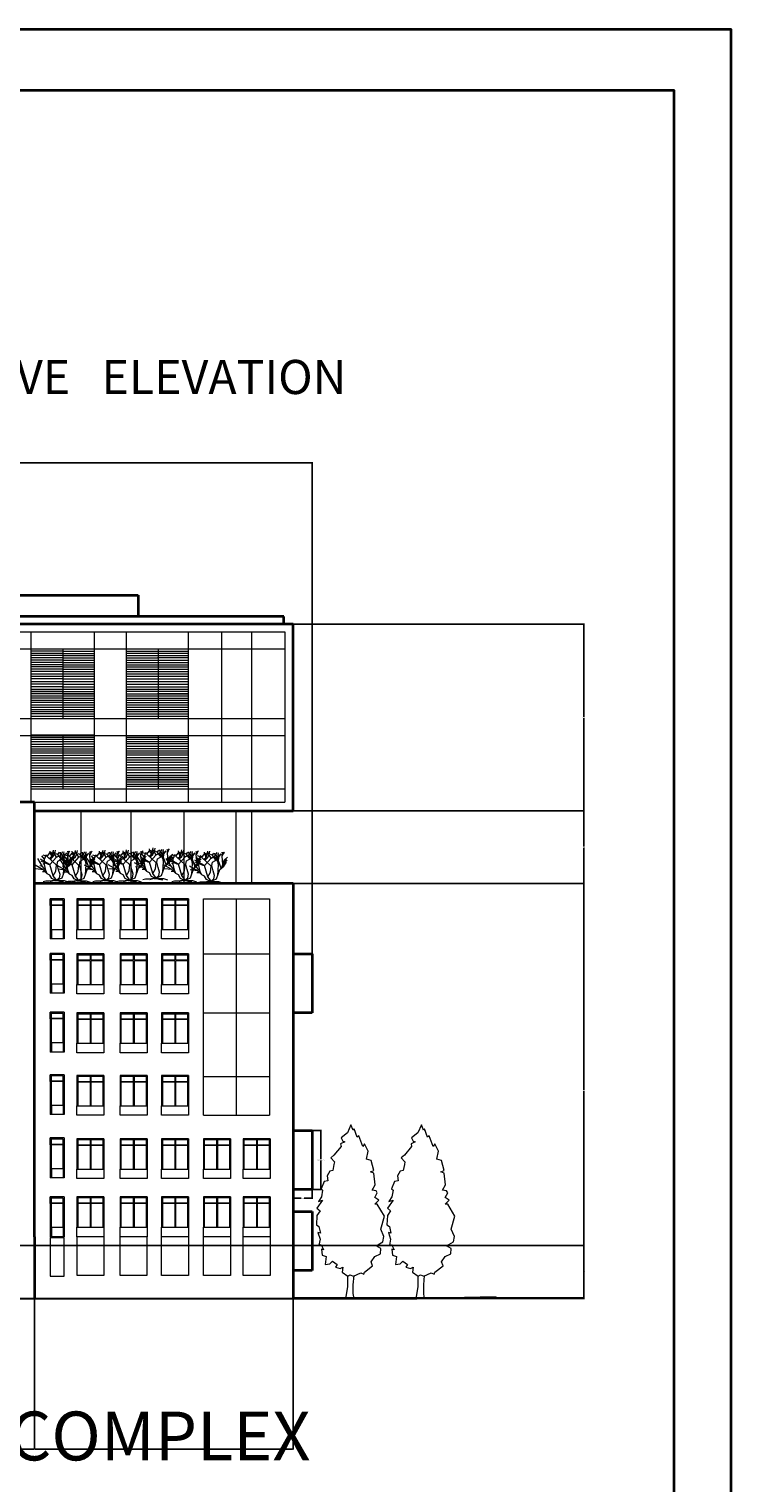
# Model space of a CAD drawing. Units: inches. Extents: x -279 to 364, y -385 to 335.
# Tile 9 of 9: x 168 to 364, y -72 to 335. Entities that reach past the tile are written whole.
import ezdxf

# ---------------------------------------------------------------- set-up
doc = ezdxf.new("R2010")
doc.units = ezdxf.units.IN
doc.header["$MEASUREMENT"] = 0
for name, color, linetype, lineweight in [('A-ANNO-DIMS', 2, 'Continuous', 18), ('A-ANNO-TEXT', 7, 'Continuous', 25), ('A-ANNO-TTLB', 7, 'Continuous', 35), ('A-GLAZ', 4, 'Continuous', 18), ('A-GLAZ-CURT', 4, 'Continuous', 18), ('A-ROOF', 7, 'Continuous', 35), ('A-WALL', 7, 'Continuous', 35), ('A-WALL-LOUV', 8, 'Continuous', 13), ('C-TOPO', 32, 'Continuous', 30), ('L-PLNT', 94, 'Continuous', 13)]:
    doc.layers.add(name, color=color, linetype=linetype, lineweight=lineweight)
doc.styles.get("Standard").update_dxf_attribs({"font": 'arial.ttf'})
doc.dimstyles.get("Standard").update_dxf_attribs({"dimtxt": 0.18, "dimasz": 0.18, "dimexe": 0.18, "dimexo": 0.0625, "dimgap": 0.09, "dimtad": 0, "dimtih": 1, "dimtoh": 1, "dimdec": 4, "dimzin": 0, "dimdsep": 46, "dimtxsty": 'Standard', "dimcen": 0.09, "dimadec": 0, "dimazin": 0, "dimtfac": 1, "dimtdec": 4, "dimtofl": 0, "dimtmove": 0, "dimatfit": 3, "dimfxl": 1, "dimtolj": 1, "dimtzin": 0, "dimarcsym": 0})

# ---------------------------------------------------------------- blocks, each defined once
blk = doc.blocks.new('*U2')
for p, q in [((-12.471, 19.775), (-12.898, 22.044)), ((-11.28, 19.619), (-12.104, 21.184)), ((-11.433, 18.289), (-10.457, 22.749)), ((-8.16, 17.76), (-10.56, 21.6)), ((-9.48, 19.775), (-8.992, 22.592)), ((-7.2, 19.68), (-6.24, 21.12)), ((-5.086, 17.741), (-5.513, 21.34)), ((-5.28, 19.2), (-3.84, 21.6)), ((-3.377, 18.602), (-2.888, 21.575)), ((-0.508, 21.888), (-0.081, 20.558)), ((-0.203, 19.149), (0.102, 21.34)), ((-0.02, 20.01), (0.896, 21.105)), ((0.041, 20.714), (1.384, 22.044)), ((0.102, 21.34), (0.835, 21.888)), ((-17.76, 8.64), (-23.663, 11.961)), ((-18.24, 11.04), (-21.755, 16.655)), ((-18.24, 11.04), (-20.16, 11.52)), ((-12.96, 12.48), (-19.68, 16.32)), ((-13.92, 12.48), (-19.2, 14.88)), ((-16.8, 16.32), (-18.72, 18.72)), ((-15.84, 8.16), (-18.24, 11.04)), ((-14.88, 18.24), (-17.76, 19.2)), ((-16.8, 12.48), (-17.76, 12.96)), ((-16.8, 16.32), (-15.36, 19.68)), ((-16.8, 12.48), (-16.8, 16.32)), ((-15.84, 8.16), (-16.8, 12.48)), ((-14.88, 18.24), (-12.96, 20.64)), ((-8.16, 12), (-14.88, 18.24)), ((-12.96, 12.48), (-13.92, 12.48)), ((-13.325, 16.724), (-11.433, 18.289)), ((-12.96, 12.48), (-8.16, 17.76)), ((-10.56, 4.32), (-12.96, 12.48)), ((-11.677, 19.071), (-12.471, 19.775)), ((-12.043, 15.628), (-11.921, 18.836)), ((-11.982, 16.802), (-10.579, 18.054)), ((-11.921, 18.836), (-10.64, 20.401)), ((-10.579, 18.054), (-9.846, 19.697)), ((-7.2, 19.68), (-8.64, 20.16)), ((-8.64, 7.68), (-8.16, 12)), ((-8.16, 17.76), (-5.28, 19.2)), ((-7.68, 12.48), (-7.2, 14.88)), ((-6.72, 8.64), (-7.68, 12.48)), ((-4.8, 16.32), (-7.2, 19.68)), ((-7.2, 14.88), (-3.84, 16.8)), ((-3.377, 15.315), (-5.086, 17.819)), ((-2.88, 12.96), (-4.32, 19.68)), ((-3.84, 16.8), (-0.96, 20.64)), ((-2.766, 16.802), (-3.377, 18.602)), ((-3.36, 5.28), (-2.88, 12.96)), ((-2.88, 15.84), (-2.4, 20.16)), ((-0.96, 10.56), (-2.88, 15.84)), ((-1.92, 9.6), (0.96, 12)), ((-0.48, 10.8), (0.346, 13.203)), ((0.346, 13.203), (-0.203, 19.149)), ((-0.142, 19.384), (0.59, 20.401)), ((0.346, 13.203), (1.323, 16.254)), ((0.96, 12), (1.44, 15.36)), ((0.96, 12), (2.88, 14.88)), ((1.323, 16.254), (3.642, 18.289)), ((1.44, 15.36), (2.88, 17.28)), ((1.92, 13.44), (2.4, 15.36)), ((2.4, 15.36), (3.36, 16.32)), ((-17.76, 8.64), (-23.128, 9.222)), ((-16.32, 7.2), (-18.24, 7.2)), ((-14.88, 5.76), (-17.76, 8.64)), ((-15.84, 0.48), (-17.76, 0)), ((-14.88, 5.76), (-15.84, 8.16)), ((-13.44, 0.48), (-15.84, 0.48)), ((-12.96, 4.8), (-14.88, 5.76)), ((-9.6, 0.96), (-13.44, 0.48)), ((-11.52, 2.4), (-12.96, 4.8)), ((-9.6, 0.96), (-12.96, 0)), ((-8.64, 0.96), (-11.52, 2.4)), ((-10.56, 4.32), (-8.64, 7.68)), ((-8.64, 1.92), (-10.56, 4.32)), ((-9.6, 0.96), (-7.68, 0.96)), ((-8.64, 0.96), (-4.32, 2.88)), ((-8.64, 0.96), (-6.24, 2.88)), ((-8.64, 0.96), (-8.64, 1.92)), ((-8.64, 0.96), (-2.88, 0.96)), ((-7.68, 0.96), (-6.24, 0.48)), ((-5.76, 5.28), (-6.72, 8.64)), ((-6.24, 2.88), (-5.76, 5.28)), ((-6.24, 0.48), (-3.36, 0)), ((-4.32, 2.88), (-1.92, 9.6)), ((-2.88, 0.96), (0, 0))]:
    blk.add_line(p, q)
blk = doc.blocks.new('*U3')
blk.add_lwpolyline([(-2.754, 191.699), (-6.78, 182.851), (-13.682, 176.953), (-11.956, 173.266), (-9.656, 172.529), (-14.257, 170.317), (-13.682, 167.368), (-21.733, 157.783), (-25.184, 154.834), (-21.158, 150.41), (-21.733, 147.461), (-22.884, 140.825), (-26.334, 140.087), (-29.21, 134.926), (-28.635, 129.028), (-32.661, 128.291), (-36.111, 120.18), (-34.386, 118.706), (-35.536, 111.333), (-38.987, 106.171), (-34.386, 107.646), (-40.712, 98.798), (-37.261, 95.849), (-40.712, 90.688), (-41.287, 80.366), (-38.412, 78.154), (-36.686, 70.781), (-39.562, 71.518), (-37.261, 64.145), (-38.412, 57.509), (-36.111, 58.247), (-33.236, 52.348), (-35.536, 53.086), (-34.961, 46.45), (-30.36, 44.975), (-31.51, 36.128), (-26.334, 36.865), (-23.459, 39.814), (-18.283, 36.128), (-20.008, 33.178), (-14.832, 31.704), (-11.956, 33.178), (-12.531, 27.28), (-6.205, 22.856), (-3.905, 24.331), (0.121, 22.856), (8.173, 26.543), (11.624, 25.068), (12.199, 27.28), (21.4, 34.653), (19.675, 39.077), (23.701, 44.975), (30.027, 47.924), (30.602, 53.823), (25.426, 56.772), (32.903, 61.196), (34.053, 67.094), (30.602, 75.205), (34.628, 89.951), (26.576, 103.222), (23.701, 103.222), (28.302, 107.646), (23.701, 110.595), (26.576, 115.756), (25.426, 117.968), (20.825, 118.706), (24.276, 124.604), (22.551, 137.876), (19.1, 139.35), (22.551, 140.825), (19.675, 151.884), (14.499, 153.359), (16.224, 162.207), (12.199, 170.317), (10.473, 167.368), (5.872, 179.165), (4.147, 177.69), (0.696, 187.275), (-0.454, 185.8)], close=True)
for points in [[(-6.813, 23.669), (-6.813, 11.669), (-8.627, 0)], [(0.387, 23.669), (-0.576, 13.271), (-0.576, 3.686), (0, 0)]]:
    blk.add_lwpolyline(points)
blk = doc.blocks.new('WIN-WING-NARROW')
for p, q in [((0, 11.12), (0, 0)), ((0, 11.12), (3.85, 11.12)), ((0.2, 2.62), (0.2, 10.81)), ((0.2, 10.81), (3.85, 10.81)), ((0.2, 9.34), (3.52, 9.34)), ((0.2, 9.24), (3.52, 9.24)), ((3.52, 9.34), (3.52, 10.81)), ((3.52, 2.62), (3.52, 9.24)), ((3.85, 9.24), (3.85, 11.12)), ((3.85, 10.81), (3.85, 9.34)), ((3.85, 9.24), (3.85, 2.62)), ((3.85, 2.62), (0, 2.62)), ((0, 0), (3.85, 0)), ((0.2, 2.62), (0.2, 0)), ((3.52, 2.62), (3.52, 0)), ((3.85, 2.62), (3.85, 0))]:
    blk.add_line(p, q)
blk = doc.blocks.new('WING-RETURN-LONG')
for p, q in [((0, 16.47), (5.32, 16.47)), ((5.32, 16.47), (5.32, 0)), ((5.32, 0), (0, 0))]:
    blk.add_line(p, q)
blk = doc.blocks.new('WIN-WING-TWIN')
for p, q in [((0, 11.12), (0, 0)), ((0, 11.12), (7.53, 11.12)), ((0.2, 2.62), (0.2, 10.81)), ((0.2, 10.81), (7.32, 10.81)), ((0.2, 9.34), (3.52, 9.34)), ((0.2, 9.24), (3.52, 9.24)), ((3.52, 9.34), (3.52, 10.81)), ((3.52, 2.62), (3.52, 9.24)), ((3.85, 10.81), (3.85, 9.34)), ((3.85, 9.34), (7.32, 9.34)), ((3.85, 9.24), (7.32, 9.24)), ((3.85, 9.24), (3.85, 2.62)), ((7.32, 10.81), (7.32, 2.62)), ((7.53, 11.12), (7.53, 2.62)), ((7.53, 2.62), (0, 2.62)), ((0, 0), (7.53, 0)), ((7.53, 0), (7.53, 2.62))]:
    blk.add_line(p, q)
blk = doc.blocks.new('*D66')
at = {"layer": 'A-ANNO-DIMS', "color": 0, "lineweight": -2, "transparency": 16777216}
for p, q in [((246.99, 26.91), (249.58, 26.91)), ((249.4, 26.73), (249.4, 18.86)), ((249.4, 10.62), (249.4, 18.49)), ((246.99, 10.44), (249.58, 10.44))]:
    blk.add_line(p, q, dxfattribs=at)
at = {"layer": 'A-ANNO-DIMS', "color": 0, "transparency": 16777216}
for points in [[(249.37, 26.73), (249.43, 26.73), (249.4, 26.91)], [(249.37, 10.62), (249.43, 10.62), (249.4, 10.44)]]:
    blk.add_solid(points, dxfattribs=at)
at = {"layer": 'Defpoints', "color": 0, "transparency": 16777216}
for p in [(246.93, 26.91), (249.4, 26.91), (246.93, 10.44)]:
    blk.add_point(p, dxfattribs=at)
at = {"layer": 'A-ANNO-DIMS', "color": 0, "transparency": 16777216, "insert": (249.4, 18.67), "char_height": 0.18, "attachment_point": 5}
blk.add_mtext('\\A1;RETURN 16 TYP.', dxfattribs=at)
blk = doc.blocks.new('*D67')
at = {"layer": 'A-ANNO-DIMS', "color": 0, "lineweight": -2, "transparency": 16777216}
for p, q in [((241.6, 10.38), (241.6, 7.79)), ((246.93, 10.38), (246.93, 7.79)), ((241.78, 7.97), (243.81, 7.97)), ((246.75, 7.97), (244.72, 7.97))]:
    blk.add_line(p, q, dxfattribs=at)
at = {"layer": 'A-ANNO-DIMS', "color": 0, "transparency": 16777216}
for points in [[(241.78, 8), (241.78, 7.94), (241.6, 7.97)], [(246.75, 8), (246.75, 7.94), (246.93, 7.97)]]:
    blk.add_solid(points, dxfattribs=at)
at = {"layer": 'Defpoints', "color": 0, "transparency": 16777216}
for p in [(241.6, 10.44), (246.93, 10.44), (246.93, 7.97)]:
    blk.add_point(p, dxfattribs=at)
at = {"layer": 'A-ANNO-DIMS', "color": 0, "transparency": 16777216, "insert": (244.26, 7.97), "char_height": 0.18, "attachment_point": 5}
blk.add_mtext('\\A1;5 TYP.', dxfattribs=at)
blk = doc.blocks.new('*D74')
at = {"layer": 'A-ANNO-DIMS', "color": 0, "lineweight": -2, "transparency": 16777216}
for p, q in [((-137.56, 76.08), (-137.56, 213.67)), ((-137.38, 213.49), (54.29, 213.49)), ((246.75, 213.49), (55.08, 213.49)), ((246.93, 76.27), (246.93, 213.67))]:
    blk.add_line(p, q, dxfattribs=at)
at = {"layer": 'A-ANNO-DIMS', "color": 0, "transparency": 16777216}
for points in [[(-137.38, 213.52), (-137.38, 213.46), (-137.56, 213.49)], [(246.75, 213.52), (246.75, 213.46), (246.93, 213.49)]]:
    blk.add_solid(points, dxfattribs=at)
at = {"layer": 'Defpoints', "color": 0, "transparency": 16777216}
for p in [(246.93, 213.49), (-137.56, 76.01), (246.93, 76.21)]:
    blk.add_point(p, dxfattribs=at)
at = {"layer": 'A-ANNO-DIMS', "color": 0, "transparency": 16777216, "insert": (54.68, 213.49), "char_height": 0.18, "attachment_point": 5}
blk.add_mtext('\\A1;384.5', dxfattribs=at)
blk = doc.blocks.new('*D80')
at = {"layer": 'A-ANNO-DIMS', "color": 0, "lineweight": -2, "transparency": 16777216}
for p, q in [((94.22, -19.95), (94.22, -62.3)), ((169.29, -19.95), (169.29, -62.3)), ((94.4, -62.12), (131.36, -62.12)), ((169.11, -62.12), (132.15, -62.12))]:
    blk.add_line(p, q, dxfattribs=at)
at = {"layer": 'A-ANNO-DIMS', "color": 0, "transparency": 16777216}
for points in [[(94.4, -62.09), (94.4, -62.15), (94.22, -62.12)], [(169.11, -62.09), (169.11, -62.15), (169.29, -62.12)]]:
    blk.add_solid(points, dxfattribs=at)
at = {"layer": 'Defpoints', "color": 0, "transparency": 16777216}
for p in [(94.22, -19.89), (169.29, -19.89), (169.29, -62.12)]:
    blk.add_point(p, dxfattribs=at)
at = {"layer": 'A-ANNO-DIMS', "color": 0, "transparency": 16777216, "insert": (131.76, -62.12), "char_height": 0.18, "attachment_point": 5}
blk.add_mtext('\\A1;75.07', dxfattribs=at)
blk = doc.blocks.new('*D81')
at = {"layer": 'A-ANNO-DIMS', "color": 0, "lineweight": -2, "transparency": 16777216}
for p, q in [((169.29, -19.95), (169.29, -62.3)), ((241.6, -19.95), (241.6, -62.3)), ((169.47, -62.12), (205.07, -62.12)), ((241.42, -62.12), (205.82, -62.12))]:
    blk.add_line(p, q, dxfattribs=at)
at = {"layer": 'A-ANNO-DIMS', "color": 0, "transparency": 16777216}
for points in [[(169.47, -62.09), (169.47, -62.15), (169.29, -62.12)], [(241.42, -62.09), (241.42, -62.15), (241.6, -62.12)]]:
    blk.add_solid(points, dxfattribs=at)
at = {"layer": 'Defpoints', "color": 0, "transparency": 16777216}
for p in [(169.29, -19.89), (241.6, -19.89), (241.6, -62.12)]:
    blk.add_point(p, dxfattribs=at)
at = {"layer": 'A-ANNO-DIMS', "color": 0, "transparency": 16777216, "insert": (205.45, -62.12), "char_height": 0.18, "attachment_point": 5}
blk.add_mtext('\\A1;72.31', dxfattribs=at)
blk = doc.blocks.new('*D82')
at = {"layer": 'A-ANNO-DIMS', "color": 0, "lineweight": -2, "transparency": 16777216}
for p, q in [((241.67, 95.9), (323.06, 95.9)), ((322.88, 95.72), (322.88, 38.19)), ((322.88, -19.71), (322.88, 37.83)), ((241.67, -19.89), (323.06, -19.89))]:
    blk.add_line(p, q, dxfattribs=at)
at = {"layer": 'A-ANNO-DIMS', "color": 0, "transparency": 16777216}
for points in [[(322.85, 95.72), (322.91, 95.72), (322.88, 95.9)], [(322.85, -19.71), (322.91, -19.71), (322.88, -19.89)]]:
    blk.add_solid(points, dxfattribs=at)
at = {"layer": 'Defpoints', "color": 0, "transparency": 16777216}
for p in [(241.6, 95.9), (322.88, 95.9), (241.6, -19.89)]:
    blk.add_point(p, dxfattribs=at)
at = {"layer": 'A-ANNO-DIMS', "color": 0, "transparency": 16777216, "insert": (322.88, 38.01), "char_height": 0.18, "attachment_point": 5}
blk.add_mtext('\\A1;115.8', dxfattribs=at)
blk = doc.blocks.new('*D83')
at = {"layer": 'A-ANNO-DIMS', "color": 0, "lineweight": -2, "transparency": 16777216}
for p, q in [((241.67, 116.19), (323.06, 116.19)), ((322.88, 116.01), (322.88, 106.23)), ((322.88, 96.08), (322.88, 105.86)), ((241.67, 95.9), (323.06, 95.9))]:
    blk.add_line(p, q, dxfattribs=at)
at = {"layer": 'A-ANNO-DIMS', "color": 0, "transparency": 16777216}
for points in [[(322.85, 116.01), (322.91, 116.01), (322.88, 116.19)], [(322.85, 96.08), (322.91, 96.08), (322.88, 95.9)]]:
    blk.add_solid(points, dxfattribs=at)
at = {"layer": 'Defpoints', "color": 0, "transparency": 16777216}
for p in [(241.6, 116.19), (322.88, 116.19), (241.6, 95.9)]:
    blk.add_point(p, dxfattribs=at)
at = {"layer": 'A-ANNO-DIMS', "color": 0, "transparency": 16777216, "insert": (322.88, 106.05), "char_height": 0.18, "attachment_point": 5}
blk.add_mtext('\\A1;20.283', dxfattribs=at)
blk = doc.blocks.new('*D84')
at = {"layer": 'A-ANNO-DIMS', "color": 0, "lineweight": -2, "transparency": 16777216}
for p, q in [((241.67, 168.38), (323.06, 168.38)), ((322.88, 168.2), (322.88, 142.47)), ((322.88, 116.37), (322.88, 142.1)), ((241.67, 116.19), (323.06, 116.19))]:
    blk.add_line(p, q, dxfattribs=at)
at = {"layer": 'A-ANNO-DIMS', "color": 0, "transparency": 16777216}
for points in [[(322.85, 168.2), (322.91, 168.2), (322.88, 168.38)], [(322.85, 116.37), (322.91, 116.37), (322.88, 116.19)]]:
    blk.add_solid(points, dxfattribs=at)
at = {"layer": 'Defpoints', "color": 0, "transparency": 16777216}
for p in [(241.6, 168.38), (322.88, 168.38), (241.6, 116.19)]:
    blk.add_point(p, dxfattribs=at)
at = {"layer": 'A-ANNO-DIMS', "color": 0, "transparency": 16777216, "insert": (322.88, 142.28), "char_height": 0.18, "attachment_point": 5}
blk.add_mtext('\\A1;52.19', dxfattribs=at)
blk = doc.blocks.new('*D96')
at = {"layer": 'A-ANNO-DIMS', "color": 0, "lineweight": -2, "transparency": 16777216}
for p, q in [((76.18, -5.23), (323.06, -5.23)), ((322.88, -5.41), (322.88, -12.47)), ((322.88, -19.9), (322.88, -12.84)), ((75.75, -20.08), (323.06, -20.08))]:
    blk.add_line(p, q, dxfattribs=at)
at = {"layer": 'A-ANNO-DIMS', "color": 0, "transparency": 16777216}
for points in [[(322.85, -5.41), (322.91, -5.41), (322.88, -5.23)], [(322.85, -19.9), (322.91, -19.9), (322.88, -20.08)]]:
    blk.add_solid(points, dxfattribs=at)
at = {"layer": 'Defpoints', "color": 0, "transparency": 16777216}
for p in [(76.12, -5.23), (322.88, -5.23), (75.69, -20.08)]:
    blk.add_point(p, dxfattribs=at)
at = {"layer": 'A-ANNO-DIMS', "color": 0, "transparency": 16777216, "insert": (322.88, -12.66), "char_height": 0.18, "attachment_point": 5}
blk.add_mtext('\\A1;14.854', dxfattribs=at)

msp = doc.modelspace()

# ---------------------------------------------------------------- linework, layer by layer
at = {"layer": 'A-ANNO-TTLB'}
for points in [[(-279.2289, 334.6468), (364.0508, 334.6468), (364.0508, -385.2219), (-279.2289, -385.2219)], [(-267.2403, 317.5778), (348.1051, 317.5778), (348.1051, -370.8321), (-267.2403, -370.8321)]]:
    msp.add_lwpolyline(points, close=True, dxfattribs=at)
at = {"layer": 'A-GLAZ'}
for p, q in [((212.1476, 41.9776), (212.3516, 41.9776)), ((173.6886, -2.9883), (177.5344, -2.9883)), ((173.6886, -2.9883), (173.6886, -13.8647)), ((177.5344, -13.8647), (177.5344, -2.9883)), ((181.173, -13.6713), (181.173, -2.7885)), ((188.7012, -2.7885), (188.7012, -13.6713)), ((193.1921, -13.6713), (193.1921, -2.7885)), ((200.7203, -2.7885), (200.7203, -13.6713)), ((204.8183, -13.6713), (204.8183, -2.7885)), ((212.3465, -2.7885), (212.3465, -13.6713)), ((216.5376, -13.6713), (216.5376, -2.7885)), ((224.0658, -2.7885), (224.0658, -13.6713)), ((227.6488, -13.6713), (227.6488, -2.7885)), ((235.177, -2.7885), (235.177, -13.6713)), ((173.6886, -13.8647), (177.5344, -13.8647)), ((177.5344, -13.8647), (177.5344, -13.8647)), ((188.7012, -13.6713), (181.173, -13.6713)), ((200.7203, -13.6713), (193.1921, -13.6713)), ((212.3465, -13.6713), (204.8183, -13.6713)), ((224.0658, -13.6713), (216.5376, -13.6713)), ((235.177, -13.6713), (227.6488, -13.6713))]:
    msp.add_line(p, q, dxfattribs=at)
at = {"layer": 'A-GLAZ-CURT'}
for p, q in [((131.2105, 166.2338), (239.2791, 166.2338)), ((168.2851, 166.2338), (168.2851, 118.6379)), ((185.9755, 166.2338), (185.9755, 118.6379)), ((194.9119, 166.2338), (194.9119, 118.6379)), ((212.2376, 166.2338), (212.2376, 118.6379)), ((221.5387, 166.2338), (221.5387, 118.6379)), ((229.928, 166.2338), (229.928, 118.6379)), ((239.2791, 166.2338), (239.2791, 118.6379)), ((131.2105, 161.4639), (239.2791, 161.4639)), ((177.2215, 161.4639), (177.2215, 150.8351)), ((203.8483, 161.4639), (203.8483, 141.986)), ((177.2215, 150.8351), (177.2215, 141.986)), ((131.2105, 141.986), (239.2791, 141.986)), ((131.2105, 137.2845), (239.2791, 137.2845)), ((177.2215, 137.3112), (177.2215, 122.2764)), ((203.8483, 137.2845), (203.8483, 122.3675)), ((185.9755, 122.3675), (239.2791, 122.3675)), ((169.2937, 118.6379), (239.2791, 118.6379)), ((182.2433, 116.1883), (182.2433, 95.9049)), ((196.215, 116.1883), (196.215, 95.9049)), ((211.0654, 116.1883), (211.0654, 95.9049)), ((225.7193, 95.9049), (225.7193, 116.1883)), ((229.9959, 116.1883), (229.9959, 95.9049)), ((216.5396, 31.1677), (216.5396, 91.5828)), ((216.5396, 91.5828), (234.973, 91.5828)), ((225.7193, 91.5828), (225.7193, 31.1677)), ((234.973, 91.5828), (234.973, 91.5828)), ((234.973, 91.5828), (234.973, 31.1677)), ((216.5396, 76.2063), (234.973, 76.2063)), ((216.5396, 59.7386), (234.973, 59.7386)), ((216.5396, 41.9776), (234.973, 41.9776)), ((216.5396, 31.1677), (234.973, 31.1677))]:
    msp.add_line(p, q, dxfattribs=at)
at = {"layer": 'A-ROOF'}
for p, q in [((140.4124, 176.4444), (198.2671, 176.4444)), ((198.2671, 176.4444), (198.2671, 170.509)), ((238.9761, 170.509), (133.5692, 170.509)), ((238.9761, 168.3808), (238.9761, 170.509))]:
    msp.add_line(p, q, dxfattribs=at)
at = {"layer": 'A-WALL'}
for p, q in [((241.6037, 168.3808), (129.2158, 168.3808)), ((241.6037, 116.1883), (241.6037, 168.3808)), ((169.2937, 118.6379), (94.2202, 118.6379)), ((169.2937, -2.7949), (169.2937, 118.6379)), ((169.2937, 116.1883), (241.6037, 116.1883)), ((176.4208, 95.9049), (169.2937, 95.9049)), ((241.6037, 95.9049), (176.4208, 95.9049)), ((241.6037, 95.9049), (241.6037, -2.4812)), ((169.2937, -2.7949), (169.2937, -19.8884)), ((241.6037, -2.4812), (241.6037, -19.8884))]:
    msp.add_line(p, q, dxfattribs=at)
at = {"layer": 'A-WALL-LOUV'}
for p, q in [((177.2215, 160.7901), (168.2851, 160.7901)), ((177.2215, 160.1684), (168.2851, 160.1684)), ((177.2215, 159.5804), (168.2851, 159.5804)), ((177.2215, 158.9482), (168.2851, 158.9482)), ((185.9779, 160.7359), (177.2215, 160.7359)), ((185.9779, 160.1142), (177.2215, 160.1142)), ((185.9779, 159.5261), (177.2215, 159.5261)), ((185.9779, 158.894), (177.2215, 158.894)), ((203.8041, 160.7466), (194.8677, 160.7466)), ((203.8041, 160.125), (194.8677, 160.125)), ((203.8041, 159.5369), (194.8677, 159.5369)), ((203.8041, 158.9047), (194.8677, 158.9047)), ((212.2376, 160.7527), (203.6648, 160.7527)), ((212.2376, 160.131), (203.6648, 160.131)), ((212.2376, 159.5429), (203.6648, 159.5429)), ((212.2376, 158.9108), (203.6648, 158.9108)), ((177.2215, 158.2695), (168.2851, 158.2695)), ((177.2215, 157.6079), (168.2851, 157.6079)), ((177.2215, 156.961), (168.2851, 156.961)), ((177.2215, 156.4024), (168.2851, 156.4024)), ((177.2215, 155.7805), (168.2851, 155.7805)), ((177.2215, 155.1017), (168.2851, 155.1017)), ((177.2215, 154.4107), (168.2851, 154.4107)), ((185.9779, 158.2153), (177.2215, 158.2153)), ((185.9779, 157.5537), (177.2215, 157.5537)), ((185.9779, 156.9068), (177.2215, 156.9068)), ((185.9779, 156.3481), (177.2215, 156.3481)), ((185.9779, 155.7263), (177.2215, 155.7263)), ((185.9779, 155.0475), (177.2215, 155.0475)), ((203.8041, 158.226), (194.8677, 158.226)), ((203.8041, 157.5644), (194.8677, 157.5644)), ((203.8041, 156.9175), (194.8677, 156.9175)), ((203.8041, 156.3589), (194.8677, 156.3589)), ((203.8041, 155.737), (194.8677, 155.737)), ((203.8041, 155.0582), (194.8677, 155.0582)), ((212.2376, 158.2321), (203.6648, 158.2321)), ((212.2376, 157.5705), (203.6648, 157.5705)), ((212.2376, 156.9236), (203.6648, 156.9236)), ((212.2376, 156.3649), (203.6648, 156.3649)), ((212.2376, 155.743), (203.6648, 155.743)), ((212.2376, 155.0643), (203.6648, 155.0643)), ((212.2376, 154.3733), (203.6648, 154.3733)), ((177.2215, 153.7491), (168.2851, 153.7491)), ((177.2215, 153.0435), (168.2851, 153.0435)), ((177.2215, 152.2643), (168.2851, 152.2643)), ((177.2215, 151.5849), (168.2851, 151.5849)), ((177.2215, 150.8351), (168.2851, 150.8351)), ((185.9779, 150.7809), (177.0415, 150.7809)), ((185.9779, 154.3565), (177.2215, 154.3565)), ((185.9779, 153.6949), (177.2215, 153.6949)), ((185.9779, 152.9892), (177.2215, 152.9892)), ((185.9779, 152.21), (177.2215, 152.21)), ((185.9779, 151.5306), (177.2215, 151.5306)), ((203.8041, 154.3672), (194.8677, 154.3672)), ((203.8041, 153.7057), (194.8677, 153.7057)), ((203.8041, 153), (194.8677, 153)), ((203.8041, 152.2208), (194.8677, 152.2208)), ((203.8041, 151.5414), (194.8677, 151.5414)), ((203.8041, 150.7916), (194.8677, 150.7916)), ((212.2376, 153.7117), (203.6648, 153.7117)), ((212.2376, 153.006), (203.6648, 153.006)), ((212.2376, 152.2268), (203.6648, 152.2268)), ((212.2376, 151.5474), (203.6648, 151.5474)), ((212.2376, 150.7976), (203.6648, 150.7976)), ((177.2215, 150.1261), (168.2851, 150.1261)), ((177.2215, 149.5528), (168.2851, 149.5528)), ((177.2215, 148.9746), (168.2851, 148.9746)), ((168.2851, 148.9567), (177.2215, 148.9567)), ((177.2215, 148.276), (168.2851, 148.276)), ((177.2215, 147.6543), (168.2851, 147.6543)), ((177.2215, 147.0663), (168.2851, 147.0663)), ((177.2215, 146.4341), (168.2851, 146.4341)), ((185.9779, 150.0719), (177.0415, 150.0719)), ((185.9779, 149.4985), (177.0415, 149.4985)), ((185.9779, 148.9203), (177.2215, 148.9203)), ((177.2215, 148.9025), (185.9779, 148.9025)), ((185.9779, 148.2218), (177.2215, 148.2218)), ((185.9779, 147.6001), (177.2215, 147.6001)), ((185.9779, 147.012), (177.2215, 147.012)), ((185.9779, 146.3799), (177.2215, 146.3799)), ((203.8041, 150.0827), (194.8677, 150.0827)), ((203.8041, 149.5093), (194.8677, 149.5093)), ((194.8677, 148.9132), (203.8041, 148.9132)), ((203.8041, 148.2325), (194.8677, 148.2325)), ((203.8041, 147.6108), (194.8677, 147.6108)), ((203.8041, 147.0228), (194.8677, 147.0228)), ((203.8041, 146.3906), (194.8677, 146.3906)), ((212.2376, 150.0887), (203.6648, 150.0887)), ((212.2376, 149.5153), (203.6648, 149.5153)), ((212.2376, 148.9371), (203.6648, 148.9371)), ((203.6648, 148.9193), (212.2376, 148.9193)), ((212.2376, 148.2385), (203.6648, 148.2385)), ((212.2376, 147.6169), (203.6648, 147.6169)), ((212.2376, 147.0288), (203.6648, 147.0288)), ((212.2376, 146.3966), (203.6648, 146.3966)), ((177.2215, 145.7554), (168.2851, 145.7554)), ((177.2215, 145.0938), (168.2851, 145.0938)), ((177.2215, 144.4469), (168.2851, 144.4469)), ((177.2215, 143.8882), (168.2851, 143.8882)), ((177.2215, 143.2664), (168.2851, 143.2664)), ((177.2215, 142.5876), (168.2851, 142.5876)), ((185.9779, 145.7011), (177.2215, 145.7011)), ((185.9779, 145.0396), (177.2215, 145.0396)), ((185.9779, 144.3927), (177.2215, 144.3927)), ((185.9779, 143.834), (177.2215, 143.834)), ((185.9779, 143.2121), (177.2215, 143.2121)), ((185.9779, 142.5334), (177.2215, 142.5334)), ((203.8041, 145.7119), (194.8677, 145.7119)), ((203.8041, 145.0503), (194.8677, 145.0503)), ((203.8041, 144.4034), (194.8677, 144.4034)), ((203.8041, 143.8448), (194.8677, 143.8448)), ((203.8041, 143.2229), (194.8677, 143.2229)), ((203.8041, 142.5441), (194.8677, 142.5441)), ((212.2376, 145.7179), (203.6648, 145.7179)), ((212.2376, 145.0564), (203.6648, 145.0564)), ((212.2376, 144.4095), (203.6648, 144.4095)), ((212.2376, 143.8508), (203.6648, 143.8508)), ((212.2376, 143.2289), (203.6648, 143.2289)), ((212.2376, 142.5502), (203.6648, 142.5502)), ((177.2165, 137.3051), (168.2801, 137.3051)), ((177.2165, 136.6835), (168.2801, 136.6835)), ((177.2165, 136.0954), (168.2801, 136.0954)), ((177.2165, 135.4632), (168.2801, 135.4632)), ((177.2165, 134.7845), (168.2801, 134.7845)), ((177.2165, 134.1229), (168.2801, 134.1229)), ((186.0136, 137.3112), (177.0772, 137.3112)), ((186.0136, 136.6895), (177.0772, 136.6895)), ((186.0136, 136.1014), (177.0772, 136.1014)), ((186.0136, 135.4693), (177.0772, 135.4693)), ((186.0136, 134.7906), (177.0772, 134.7906)), ((186.0136, 134.129), (177.0772, 134.129)), ((203.9408, 136.7347), (195.0045, 136.7347)), ((203.9408, 136.113), (195.0045, 136.113)), ((203.9408, 135.5249), (195.0045, 135.5249)), ((203.9408, 134.8928), (195.0045, 134.8928)), ((203.9408, 134.2141), (195.0045, 134.2141)), ((212.2376, 136.7407), (203.8016, 136.7407)), ((212.2376, 136.1191), (203.8016, 136.1191)), ((212.2376, 135.531), (203.8016, 135.531)), ((212.2376, 134.8988), (203.8016, 134.8988)), ((212.2376, 134.2201), (203.8016, 134.2201)), ((177.2165, 133.476), (168.2801, 133.476)), ((177.2165, 132.9174), (168.2801, 132.9174)), ((177.2165, 132.2955), (168.2801, 132.2955)), ((177.2165, 131.6167), (168.2801, 131.6167)), ((177.2165, 130.9257), (168.2801, 130.9257)), ((177.2165, 130.2642), (168.2801, 130.2642)), ((186.0136, 133.4821), (177.0772, 133.4821)), ((186.0136, 132.9234), (177.0772, 132.9234)), ((186.0136, 132.3015), (177.0772, 132.3015)), ((186.0136, 131.6228), (177.0772, 131.6228)), ((186.0136, 130.9318), (177.0772, 130.9318)), ((186.0136, 130.2702), (177.0772, 130.2702)), ((203.9408, 133.5525), (195.0045, 133.5525)), ((203.9408, 132.9056), (195.0045, 132.9056)), ((203.9408, 132.3469), (195.0045, 132.3469)), ((203.9408, 131.7251), (195.0045, 131.7251)), ((203.9408, 131.0463), (195.0045, 131.0463)), ((203.9408, 130.3553), (195.0045, 130.3553)), ((212.2376, 133.5585), (203.8016, 133.5585)), ((212.2376, 132.9116), (203.8016, 132.9116)), ((212.2376, 132.353), (203.8016, 132.353)), ((212.2376, 131.7311), (203.8016, 131.7311)), ((212.2376, 131.0523), (203.8016, 131.0523)), ((212.2376, 130.3613), (203.8016, 130.3613)), ((177.2165, 129.5585), (168.2801, 129.5585)), ((177.2165, 128.7793), (168.2801, 128.7793)), ((177.2165, 128.0999), (168.2801, 128.0999)), ((177.2165, 127.3501), (168.2801, 127.3501)), ((177.2165, 126.6412), (168.2801, 126.6412)), ((177.2165, 126.0678), (168.2801, 126.0678)), ((186.0136, 129.5645), (177.0772, 129.5645)), ((186.0136, 128.7853), (177.0772, 128.7853)), ((186.0136, 128.1059), (177.0772, 128.1059)), ((186.0136, 127.3561), (177.0772, 127.3561)), ((186.0136, 126.6472), (177.0772, 126.6472)), ((186.0136, 126.0738), (177.0772, 126.0738)), ((203.9408, 129.6937), (195.0045, 129.6937)), ((203.9408, 128.988), (195.0045, 128.988)), ((203.9408, 128.2088), (195.0045, 128.2088)), ((203.9408, 127.5294), (195.0045, 127.5294)), ((203.9408, 126.7796), (195.0045, 126.7796)), ((203.9408, 126.0707), (195.0045, 126.0707)), ((212.2376, 129.6998), (203.8016, 129.6998)), ((212.2376, 128.9941), (203.8016, 128.9941)), ((212.2376, 128.2149), (203.8016, 128.2149)), ((212.2376, 127.5355), (203.8016, 127.5355)), ((212.2376, 126.7857), (203.8016, 126.7857)), ((212.2376, 126.0768), (203.8016, 126.0768)), ((177.2165, 125.4896), (168.2801, 125.4896)), ((168.2801, 125.4717), (177.2165, 125.4717)), ((177.2165, 124.791), (168.2801, 124.791)), ((177.2165, 124.1693), (168.2801, 124.1693)), ((177.2165, 123.5813), (168.2801, 123.5813)), ((177.2165, 122.9491), (168.2801, 122.9491)), ((177.2165, 122.2704), (168.2801, 122.2704)), ((186.0136, 125.4956), (177.0772, 125.4956)), ((177.0772, 125.4778), (186.0136, 125.4778)), ((186.0136, 124.797), (177.0772, 124.797)), ((186.0136, 124.1754), (177.0772, 124.1754)), ((186.0136, 123.5873), (177.0772, 123.5873)), ((186.0136, 122.9551), (177.0772, 122.9551)), ((186.0136, 122.2764), (177.0772, 122.2764)), ((203.9408, 125.4973), (195.0045, 125.4973)), ((203.9408, 124.9191), (195.0045, 124.9191)), ((195.0045, 124.9013), (203.9408, 124.9013)), ((203.9408, 124.2206), (195.0045, 124.2206)), ((203.9408, 123.5989), (195.0045, 123.5989)), ((203.9408, 123.0108), (195.0045, 123.0108)), ((212.2376, 125.5034), (203.8016, 125.5034)), ((212.2376, 124.9252), (203.8016, 124.9252)), ((203.8016, 124.9073), (212.2376, 124.9073)), ((212.2376, 124.2266), (203.8016, 124.2266)), ((212.2376, 123.605), (203.8016, 123.605)), ((212.2376, 123.0169), (203.8016, 123.0169)), ((168.2851, 121.6088), (168.2801, 121.6088)), ((168.2851, 120.9619), (168.2801, 120.9619)), ((168.2851, 120.4033), (168.2801, 120.4033)), ((168.2851, 119.7814), (168.2801, 119.7814)), ((168.2851, 119.1026), (168.2801, 119.1026))]:
    msp.add_line(p, q, dxfattribs=at)
at = {"layer": 'C-TOPO'}
for p, q in [((-133.7987, -20.0818), (198.4631, -20.0818)), ((31.9982, -20.0818), (198.4631, -20.0818)), ((198.4631, -20.0818), (276.2424, -20.0818)), ((276.2424, -20.0818), (298.3779, -19.592))]:
    msp.add_line(p, q, dxfattribs=at)

# ---------------------------------------------------------------- block references
at = {"layer": 'A-GLAZ', "extrusion": (0, 0, -1), "zscale": -1}
for name, p in [('WIN-WING-NARROW', (-177.531, 80.4674)), ('WIN-WING-TWIN', (-188.6751, 80.4674)), ('WIN-WING-TWIN', (-200.7574, 80.4674)), ('WIN-WING-TWIN', (-212.3516, 80.4674)), ('WIN-WING-NARROW', (-177.531, 65.2654)), ('WIN-WING-TWIN', (-188.6751, 65.0909)), ('WIN-WING-TWIN', (-200.7574, 65.0909)), ('WIN-WING-TWIN', (-212.3516, 65.0909)), ('WIN-WING-NARROW', (-177.531, 48.8069)), ('WIN-WING-TWIN', (-188.6751, 48.6233)), ('WIN-WING-TWIN', (-200.7574, 48.6233)), ('WIN-WING-TWIN', (-212.3516, 48.6233)), ('WIN-WING-NARROW', (-177.531, 31.3188)), ('WIN-WING-TWIN', (-188.6751, 31.1677)), ('WIN-WING-TWIN', (-200.7574, 31.1677)), ('WIN-WING-TWIN', (-212.3516, 31.1677)), ('WIN-WING-NARROW', (-177.531, 13.6747)), ('WIN-WING-TWIN', (-188.6751, 13.4768)), ('WIN-WING-TWIN', (-200.7574, 13.4768)), ('WIN-WING-TWIN', (-212.3516, 13.4768)), ('WIN-WING-TWIN', (-224.0678, 13.4768)), ('WIN-WING-TWIN', (-235.177, 13.4768)), ('WIN-WING-NARROW', (-177.531, -2.7949)), ('WIN-WING-TWIN', (-188.6751, -2.7886)), ('WIN-WING-TWIN', (-200.7574, -2.7886)), ('WIN-WING-TWIN', (-212.3516, -2.7886)), ('WIN-WING-TWIN', (-224.0678, -2.7886)), ('WIN-WING-TWIN', (-235.177, -2.7886))]:
    msp.add_blockref(name, p, dxfattribs=at)
at = {"layer": 'A-WALL'}
for p in [(241.604, 59.739), (241.604, 10.4405), (241.604, -12.2083)]:
    msp.add_blockref('WING-RETURN-LONG', p, dxfattribs=at)
at = {"layer": 'L-PLNT'}
for name, p, xscale, yscale, zscale in [('*U2', (206.5196, 96.9652), 0.390298493085325, 0.390298493085325, 0.390298493085325), ('*U2', (178.6598, 96.3663), 0.390298493085325, 0.390298493085325, 0.390298493085325), ('*U2', (184.8413, 96.2861), 0.390298493085325, 0.390298493085325, 0.390298493085325), ('*U2', (192.5224, 96.3663), 0.390298493085325, 0.390298493085325, 0.390298493085325), ('*U2', (199.1173, 96.4031), 0.390298493085325, 0.390298493085325, 0.390298493085325), ('*U2', (214.595, 96.4031), 0.390298493085325, 0.390298493085325, 0.390298493085325), ('*U2', (221.8377, 96.0904), 0.390298493085325, 0.390298493085325, 0.390298493085325), ('*U3', (258.4788, -19.592), 0.2508480261805224, 0.2508480261805224, 0.2508480261805224), ('*U3', (278.1686, -19.592), 0.2508480261805224, 0.2508480261805224, 0.2508480261805224)]:
    msp.add_blockref(name, p, dxfattribs=dict(at, xscale=xscale, yscale=yscale, zscale=zscale))

# ---------------------------------------------------------------- texts
at = {"layer": 'A-ANNO-TEXT'}
for s, height, p in [('MEGA   SCALE   INSTITUTIONAL   CAMPUS   COMPREHENSIVE   ELEVATION ', 9.539438, (-183.0703, 232.6637)), ('FRONT   ELEVATION   MAIN   ACADEMIC   COMPLEX', 13.648689, (-182.5362, -65.301))]:
    msp.add_text(s, height=height, dxfattribs=at).set_placement(p)

# ---------------------------------------------------------------- dimensions: what is measured, and where the dimension line sits
at = {"layer": 'A-ANNO-DIMS'}
for base, p1, p2, override, picture, middle in [((246.9255, 213.4896), (-137.5587, 76.0128), (246.9255, 76.2063), {"dimdec": 1, "dimlfac": 1, "dimrnd": 0, "dimzin": 0, "dimdsep": 46, "dimlunit": 2}, '*D74', (54.6834, 213.4896)), ((169.2937, -62.1247), (94.2202, -19.8884), (169.2937, -19.8884), {"dimdec": 2, "dimlfac": 1, "dimrnd": 0, "dimzin": 0, "dimdsep": 46, "dimlunit": 2}, '*D80', (131.757, -62.1247)), ((241.6037, -62.1247), (169.2937, -19.8884), (241.6037, -19.8884), {"dimdec": 2, "dimlfac": 1, "dimrnd": 0, "dimzin": 0, "dimdsep": 46, "dimlunit": 2}, '*D81', (205.4487, -62.1247))]:
    dim = msp.add_linear_dim(base=base, p1=p1, p2=p2, dimstyle='Standard', override=override, dxfattribs=at)
    dim.commit()
    dim.dimension.update_dxf_attribs({"geometry": picture, "text_midpoint": middle})
for base, p1, p2, override, picture, middle in [((322.8779, 168.3808), (241.6037, 116.1883), (241.6037, 168.3808), {"dimdec": 2, "dimlfac": 1, "dimrnd": 0, "dimzin": 0, "dimdsep": 46, "dimlunit": 2}, '*D84', (322.8779, 142.2846)), ((322.8779, 116.1883), (241.6037, 95.9049), (241.6037, 116.1883), {"dimdec": 3, "dimlfac": 1, "dimrnd": 0, "dimzin": 0, "dimdsep": 46, "dimlunit": 2}, '*D83', (322.8779, 106.0466)), ((322.8779, 95.9049), (241.6037, -19.8884), (241.6037, 95.9049), {"dimdec": 1, "dimlfac": 1, "dimrnd": 0, "dimzin": 0, "dimdsep": 46, "dimlunit": 2}, '*D82', (322.8779, 38.0082)), ((322.8779, -5.2282), (75.6857, -20.0818), (76.1172, -5.2282), {"dimdec": 3, "dimlfac": 1, "dimrnd": 0, "dimzin": 0, "dimdsep": 46, "dimlunit": 2}, '*D96', (322.8779, -12.655))]:
    dim = msp.add_linear_dim(base=base, p1=p1, p2=p2, angle=90, dimstyle='Standard', override=override, dxfattribs=at)
    dim.commit()
    dim.dimension.update_dxf_attribs({"geometry": picture, "text_midpoint": middle})
dim = msp.add_linear_dim(base=(249.3957, 26.9078), p1=(246.9255, 10.4402), p2=(246.9255, 26.9078), angle=90, text='RETURN <> TYP.', dimstyle='Standard', override={"dimdec": 0, "dimlfac": 1, "dimrnd": 0, "dimzin": 0, "dimdsep": 46, "dimlunit": 2}, dxfattribs=at)
dim.commit()
dim.dimension.update_dxf_attribs({"geometry": '*D66', "text_midpoint": (249.3957, 18.674)})
dim = msp.add_linear_dim(base=(246.9255, 7.97), p1=(241.6037, 10.4402), p2=(246.9255, 10.4402), text='<> TYP.', dimstyle='Standard', override={"dimdec": 0, "dimlfac": 1, "dimrnd": 0, "dimzin": 0, "dimdsep": 46, "dimlunit": 2}, dxfattribs=at)
dim.commit()
dim.dimension.update_dxf_attribs({"geometry": '*D67', "text_midpoint": (244.2646, 7.97)})

doc.saveas('drawing.dxf')
